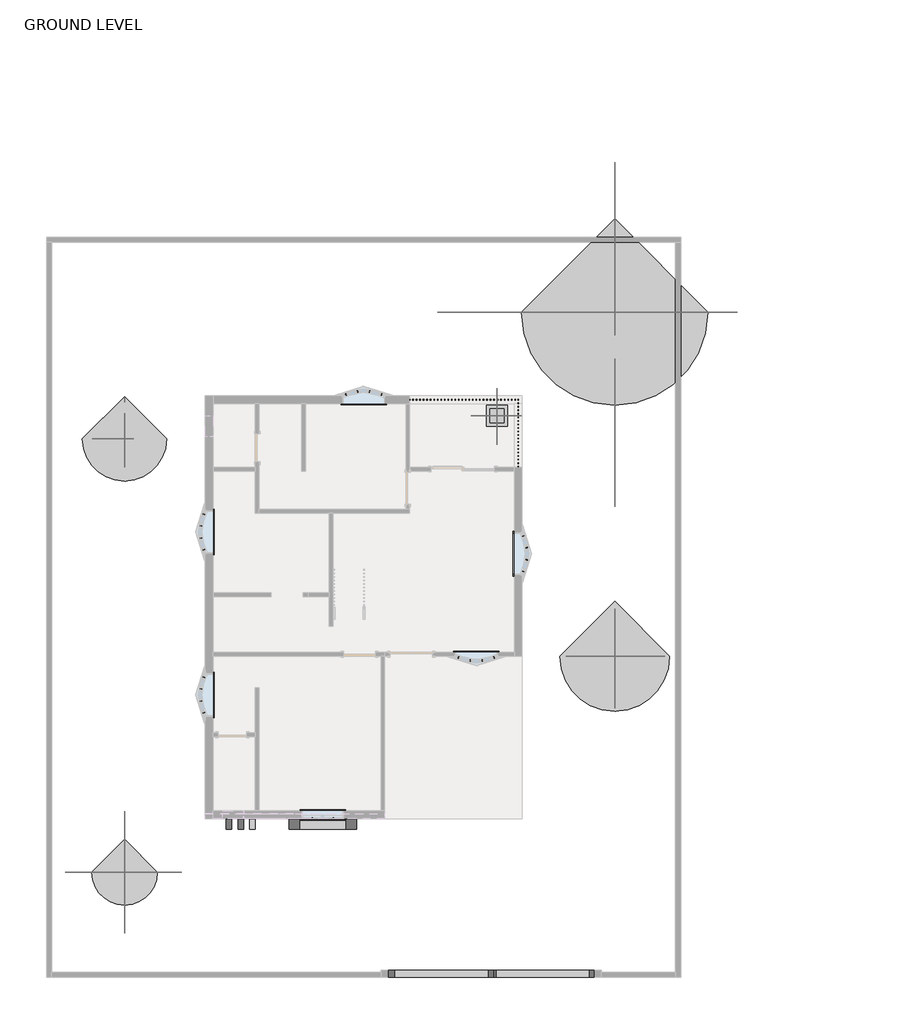
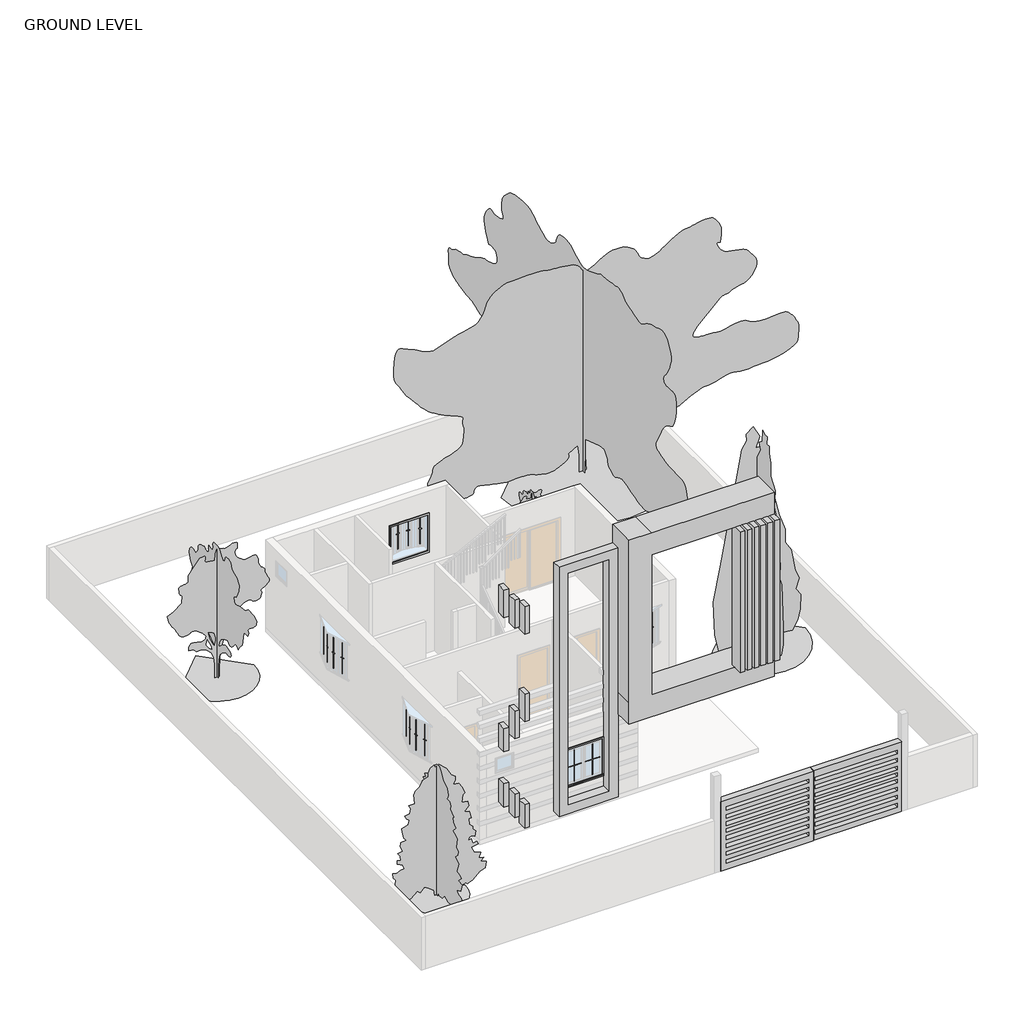
# One storey, part 3 of 3: 30 proxies, 6 geographic elements, 1 railing.
"""IFC4 building model written with IfcOpenShell, lengths in millimetres."""

from ifc_helpers import new_model, si_unit, frame, origin, place, context, project, spatial, polyline, outline, extrude, faceted_brep, transform, mapped, element, save
from components import generic_models_1_generic_models_1_2996b52b, muntin_pattern_2x2_muntin_pattern_2x2_750a293b, muntin_pattern_2x2_muntin_pattern_2x2_a9af9031, muntin_pattern_2x2_muntin_pattern_2x2_4dfeb3f3, muntin_pattern_2x2_muntin_pattern_2x2_e852a7e4, trim_window_exterior_flat_with_sill_7cfdd449, trim_window_interior_flat_picture_frame_ace0ae79, trim_window_interior_flat_picture_frame_f1e0b15b, planter_2_x2_da431093, rpc_tree_conifer_9825e489, rpc_tree_conifer_red_cedar_10_2_15f97043, rpc_tree_deciduous_15_10e6bd9b, rpc_tree_deciduous_japanese_cherry_15_720dba75, rpc_tree_deciduous_japanese_cherry_15_2_e499737d

model = new_model("IFC4")

# Units and contexts
model_context = context("Model", 3, world=origin())
ifc_project = project(units=[si_unit("LENGTHUNIT", "METRE", prefix="MILLI")], contexts=[model_context])

# Site, building, storey
site = spatial("IfcSite", under=ifc_project)
building = spatial("IfcBuilding", under=site)
storey = spatial("IfcBuildingStorey", under=building, Name="GROUND LEVEL", Elevation=0.0)

# Proxies
placement = place(None, origin())
generic_models_1_generic_models_1_shape = generic_models_1_generic_models_1_2996b52b(model_context)
element("IfcBuildingElementProxy", 1, Name="Generic Models 1 : Generic Models 1", ObjectType="Generic Models 1 : Generic Models 1", at=placement, inside=storey, context=model_context, shape_type="MappedRepresentation", body=[
    mapped(generic_models_1_generic_models_1_shape, transform((0.0, 0.0, 0.0), x_axis=(1.0, 0.0, 0.0), y_axis=(0.0, 1.0, 0.0), z_axis=(0.0, 0.0, 1.0))),
])
muntin_pattern_2x2_muntin_pattern_2x2_shape = muntin_pattern_2x2_muntin_pattern_2x2_750a293b(model_context)
element("IfcBuildingElementProxy", 2, Name="Muntin Pattern_2x2 : Muntin Pattern_2x2", ObjectType="Muntin Pattern_2x2 : Muntin Pattern_2x2", at=placement, inside=storey, context=model_context, shape_type="MappedRepresentation", body=[
    mapped(muntin_pattern_2x2_muntin_pattern_2x2_shape, transform((2505.3380176, -905.714627, 1114.3823709), x_axis=(-0.9396926207859141, -0.3420201433256534, 0.0), y_axis=(0.3420201433256534, -0.9396926207859141, 0.0), z_axis=(0.0, 0.0, 1.0))),
])
element("IfcBuildingElementProxy", 3, Name="Muntin Pattern_2x2 : Muntin Pattern_2x2", ObjectType="Muntin Pattern_2x2 : Muntin Pattern_2x2", at=placement, inside=storey, context=model_context, shape_type="MappedRepresentation", body=[
    mapped(muntin_pattern_2x2_muntin_pattern_2x2_shape, transform((1482.0289314, -905.714627, 1114.3823709), x_axis=(-0.939692620785903, 0.34202014332568337, 0.0), y_axis=(-0.34202014332568337, -0.939692620785903, 0.0), z_axis=(0.0, 0.0, 1.0))),
])
element("IfcBuildingElementProxy", 4, Name="Muntin Pattern_2x2 : Muntin Pattern_2x2", ObjectType="Muntin Pattern_2x2 : Muntin Pattern_2x2", at=placement, inside=storey, context=model_context, shape_type="MappedRepresentation", body=[
    mapped(muntin_pattern_2x2_muntin_pattern_2x2_shape, transform((2166.3285145, -996.5519495, 1114.3823709), x_axis=(-0.9848077530122118, -0.17364817766690924, 0.0), y_axis=(0.17364817766690924, -0.9848077530122118, 0.0), z_axis=(0.0, 0.0, 1.0))),
])
element("IfcBuildingElementProxy", 5, Name="Muntin Pattern_2x2 : Muntin Pattern_2x2", ObjectType="Muntin Pattern_2x2 : Muntin Pattern_2x2", at=placement, inside=storey, context=model_context, shape_type="MappedRepresentation", body=[
    mapped(muntin_pattern_2x2_muntin_pattern_2x2_shape, transform((-5861.4497338, -2499.7623237, 1114.3823709), x_axis=(-0.342020143325655, 0.9396926207859135, 0.0), y_axis=(-0.9396926207859135, -0.342020143325655, 0.0), z_axis=(0.0, 0.0, 1.0))),
])
element("IfcBuildingElementProxy", 6, Name="Muntin Pattern_2x2 : Muntin Pattern_2x2", ObjectType="Muntin Pattern_2x2 : Muntin Pattern_2x2", at=placement, inside=storey, context=model_context, shape_type="MappedRepresentation", body=[
    mapped(muntin_pattern_2x2_muntin_pattern_2x2_shape, transform((-5861.4497338, -1476.4532375, 1114.3823709), x_axis=(0.34202014332568176, 0.9396926207859035, 0.0), y_axis=(-0.9396926207859035, 0.34202014332568176, 0.0), z_axis=(0.0, 0.0, 1.0))),
])
element("IfcBuildingElementProxy", 7, Name="Muntin Pattern_2x2 : Muntin Pattern_2x2", ObjectType="Muntin Pattern_2x2 : Muntin Pattern_2x2", at=placement, inside=storey, context=model_context, shape_type="MappedRepresentation", body=[
    mapped(muntin_pattern_2x2_muntin_pattern_2x2_shape, transform((-5952.2870564, -2160.7528206, 1114.3823709), x_axis=(-0.1736481776669109, 0.9848077530122115, 0.0), y_axis=(-0.9848077530122115, -0.1736481776669109, 0.0), z_axis=(0.0, 0.0, 1.0))),
])
element("IfcBuildingElementProxy", 8, Name="Muntin Pattern_2x2 : Muntin Pattern_2x2", ObjectType="Muntin Pattern_2x2 : Muntin Pattern_2x2", at=placement, inside=storey, context=model_context, shape_type="MappedRepresentation", body=[
    mapped(muntin_pattern_2x2_muntin_pattern_2x2_shape, transform((-1766.8960515, 6668.4018239, 1114.3823709), x_axis=(0.9396926207859141, 0.3420201433256534, 0.0), y_axis=(-0.3420201433256534, 0.9396926207859141, 0.0), z_axis=(0.0, 0.0, 1.0))),
])
element("IfcBuildingElementProxy", 9, Name="Muntin Pattern_2x2 : Muntin Pattern_2x2", ObjectType="Muntin Pattern_2x2 : Muntin Pattern_2x2", at=placement, inside=storey, context=model_context, shape_type="MappedRepresentation", body=[
    mapped(muntin_pattern_2x2_muntin_pattern_2x2_shape, transform((-743.5869653, 6668.4018239, 1114.3823709), x_axis=(0.939692620785903, -0.34202014332568337, 0.0), y_axis=(0.34202014332568337, 0.939692620785903, 0.0), z_axis=(0.0, 0.0, 1.0))),
])
element("IfcBuildingElementProxy", 10, Name="Muntin Pattern_2x2 : Muntin Pattern_2x2", ObjectType="Muntin Pattern_2x2 : Muntin Pattern_2x2", at=placement, inside=storey, context=model_context, shape_type="MappedRepresentation", body=[
    mapped(muntin_pattern_2x2_muntin_pattern_2x2_shape, transform((-1427.8865484, 6759.2391465, 1114.3823709), x_axis=(0.9848077530122118, 0.1736481776669092, 0.0), y_axis=(-0.1736481776669092, 0.9848077530122118, 0.0), z_axis=(0.0, 0.0, 1.0))),
])
element("IfcBuildingElementProxy", 11, Name="Muntin Pattern_2x2 : Muntin Pattern_2x2", ObjectType="Muntin Pattern_2x2 : Muntin Pattern_2x2", at=placement, inside=storey, context=model_context, shape_type="MappedRepresentation", body=[
    mapped(muntin_pattern_2x2_muntin_pattern_2x2_shape, transform((-5861.4497338, 2196.9198574, 1114.3823709), x_axis=(-0.342020143325655, 0.9396926207859135, 0.0), y_axis=(-0.9396926207859135, -0.342020143325655, 0.0), z_axis=(0.0, 0.0, 1.0))),
])
element("IfcBuildingElementProxy", 12, Name="Muntin Pattern_2x2 : Muntin Pattern_2x2", ObjectType="Muntin Pattern_2x2 : Muntin Pattern_2x2", at=placement, inside=storey, context=model_context, shape_type="MappedRepresentation", body=[
    mapped(muntin_pattern_2x2_muntin_pattern_2x2_shape, transform((-5861.4497338, 3220.2289436, 1114.3823709), x_axis=(0.34202014332568176, 0.9396926207859035, 0.0), y_axis=(-0.9396926207859035, 0.34202014332568176, 0.0), z_axis=(0.0, 0.0, 1.0))),
])
element("IfcBuildingElementProxy", 13, Name="Muntin Pattern_2x2 : Muntin Pattern_2x2", ObjectType="Muntin Pattern_2x2 : Muntin Pattern_2x2", at=placement, inside=storey, context=model_context, shape_type="MappedRepresentation", body=[
    mapped(muntin_pattern_2x2_muntin_pattern_2x2_shape, transform((-5952.2870564, 2535.9293605, 1114.3823709), x_axis=(-0.1736481776669109, 0.9848077530122115, 0.0), y_axis=(-0.9848077530122115, -0.1736481776669109, 0.0), z_axis=(0.0, 0.0, 1.0))),
])
element("IfcBuildingElementProxy", 14, Name="Muntin Pattern_2x2 : Muntin Pattern_2x2", ObjectType="Muntin Pattern_2x2 : Muntin Pattern_2x2", at=placement, inside=storey, context=model_context, shape_type="MappedRepresentation", body=[
    mapped(muntin_pattern_2x2_muntin_pattern_2x2_shape, transform((3350.9667171, 2592.8981416, 730.25), x_axis=(0.34202014332565495, -0.9396926207859135, 0.0), y_axis=(0.9396926207859135, 0.34202014332565495, 0.0), z_axis=(0.0, 0.0, 1.0))),
])
element("IfcBuildingElementProxy", 15, Name="Muntin Pattern_2x2 : Muntin Pattern_2x2", ObjectType="Muntin Pattern_2x2 : Muntin Pattern_2x2", at=placement, inside=storey, context=model_context, shape_type="MappedRepresentation", body=[
    mapped(muntin_pattern_2x2_muntin_pattern_2x2_shape, transform((3350.9667171, 1569.5890554, 730.25), x_axis=(-0.3420201433256818, -0.9396926207859035, 0.0), y_axis=(0.9396926207859035, -0.3420201433256818, 0.0), z_axis=(0.0, 0.0, 1.0))),
])
element("IfcBuildingElementProxy", 16, Name="Muntin Pattern_2x2 : Muntin Pattern_2x2", ObjectType="Muntin Pattern_2x2 : Muntin Pattern_2x2", at=placement, inside=storey, context=model_context, shape_type="MappedRepresentation", body=[
    mapped(muntin_pattern_2x2_muntin_pattern_2x2_shape, transform((3441.8040397, 2253.8886385, 730.25), x_axis=(0.17364817766691085, -0.9848077530122115, 0.0), y_axis=(0.9848077530122115, 0.17364817766691085, 0.0), z_axis=(0.0, 0.0, 1.0))),
])
muntin_pattern_2x2_muntin_pattern_2x2_2_shape = muntin_pattern_2x2_muntin_pattern_2x2_a9af9031(model_context)
element("IfcBuildingElementProxy", 17, Name="Muntin Pattern_2x2 : Muntin Pattern_2x2", ObjectType="Muntin Pattern_2x2 : Muntin Pattern_2x2", at=placement, inside=storey, context=model_context, shape_type="MappedRepresentation", body=[
    mapped(muntin_pattern_2x2_muntin_pattern_2x2_2_shape, transform((1821.0384345, -996.5519495, 1114.3823709), x_axis=(0.9848077530122107, -0.17364817766691557, 0.0), y_axis=(0.17364817766691557, 0.9848077530122107, 0.0), z_axis=(0.0, 0.0, 1.0))),
])
element("IfcBuildingElementProxy", 18, Name="Muntin Pattern_2x2 : Muntin Pattern_2x2", ObjectType="Muntin Pattern_2x2 : Muntin Pattern_2x2", at=placement, inside=storey, context=model_context, shape_type="MappedRepresentation", body=[
    mapped(muntin_pattern_2x2_muntin_pattern_2x2_2_shape, transform((-5952.2870564, -1815.4627406, 1114.3823709), x_axis=(-0.1736481776669139, -0.984807753012211, 0.0), y_axis=(0.984807753012211, -0.1736481776669139, 0.0), z_axis=(0.0, 0.0, 1.0))),
])
element("IfcBuildingElementProxy", 19, Name="Muntin Pattern_2x2 : Muntin Pattern_2x2", ObjectType="Muntin Pattern_2x2 : Muntin Pattern_2x2", at=placement, inside=storey, context=model_context, shape_type="MappedRepresentation", body=[
    mapped(muntin_pattern_2x2_muntin_pattern_2x2_2_shape, transform((-1082.5964684, 6759.2391465, 1114.3823709), x_axis=(-0.9848077530122107, 0.1736481776669156, 0.0), y_axis=(-0.1736481776669156, -0.9848077530122107, 0.0), z_axis=(0.0, 0.0, 1.0))),
])
element("IfcBuildingElementProxy", 20, Name="Muntin Pattern_2x2 : Muntin Pattern_2x2", ObjectType="Muntin Pattern_2x2 : Muntin Pattern_2x2", at=placement, inside=storey, context=model_context, shape_type="MappedRepresentation", body=[
    mapped(muntin_pattern_2x2_muntin_pattern_2x2_2_shape, transform((-5952.2870564, 2881.2194405, 1114.3823709), x_axis=(-0.1736481776669139, -0.984807753012211, 0.0), y_axis=(0.984807753012211, -0.1736481776669139, 0.0), z_axis=(0.0, 0.0, 1.0))),
])
element("IfcBuildingElementProxy", 21, Name="Muntin Pattern_2x2 : Muntin Pattern_2x2", ObjectType="Muntin Pattern_2x2 : Muntin Pattern_2x2", at=placement, inside=storey, context=model_context, shape_type="MappedRepresentation", body=[
    mapped(muntin_pattern_2x2_muntin_pattern_2x2_2_shape, transform((3441.8040397, 1908.5985585, 730.25), x_axis=(0.17364817766691396, 0.984807753012211, 0.0), y_axis=(-0.984807753012211, 0.17364817766691396, 0.0), z_axis=(0.0, 0.0, 1.0))),
])
muntin_pattern_2x2_muntin_pattern_2x2_3_shape = muntin_pattern_2x2_muntin_pattern_2x2_4dfeb3f3(model_context)
element("IfcBuildingElementProxy", 22, Name="Muntin Pattern_2x2 : Muntin Pattern_2x2", ObjectType="Muntin Pattern_2x2 : Muntin Pattern_2x2", at=placement, inside=storey, context=model_context, shape_type="MappedRepresentation", body=[
    mapped(muntin_pattern_2x2_muntin_pattern_2x2_3_shape, transform((-2130.1595223, -5548.2814015, 984.25), x_axis=(-1.0, 0.0, 0.0), y_axis=(0.0, -1.0, 0.0), z_axis=(0.0, 0.0, 1.0))),
])
muntin_pattern_2x2_muntin_pattern_2x2_4_shape = muntin_pattern_2x2_muntin_pattern_2x2_e852a7e4(model_context)
element("IfcBuildingElementProxy", 23, Name="Muntin Pattern_2x2 : Muntin Pattern_2x2", ObjectType="Muntin Pattern_2x2 : Muntin Pattern_2x2", at=placement, inside=storey, context=model_context, shape_type="MappedRepresentation", body=[
    mapped(muntin_pattern_2x2_muntin_pattern_2x2_4_shape, transform((-2736.5845223, -5548.2814015, 984.25), x_axis=(1.0, 0.0, 0.0), y_axis=(0.0, 1.0, 0.0), z_axis=(0.0, 0.0, 1.0))),
])
trim_window_exterior_flat_with_sill_shape = trim_window_exterior_flat_with_sill_7cfdd449(model_context)
element("IfcBuildingElementProxy", 24, Name="Trim-Window-Exterior-Flat : with Sill", ObjectType="Trim-Window-Exterior-Flat : with Sill", at=placement, inside=storey, context=model_context, shape_type="MappedRepresentation", body=[
    mapped(trim_window_exterior_flat_with_sill_shape, transform((-2433.3720223, -5557.8064015, 2133.6), x_axis=(1.0, 0.0, 0.0), y_axis=(0.0, 0.0, 1.0), z_axis=(0.0, -1.0, 0.0))),
])
trim_window_interior_flat_picture_frame_shape = trim_window_interior_flat_picture_frame_ace0ae79(model_context)
element("IfcBuildingElementProxy", 25, Name="Trim-Window-Interior-Flat : Picture Frame", ObjectType="Trim-Window-Interior-Flat : Picture Frame", at=placement, inside=storey, context=model_context, shape_type="MappedRepresentation", body=[
    mapped(trim_window_interior_flat_picture_frame_shape, transform((1993.6834745, -757.2064015, 2263.7323709), x_axis=(-1.0, 0.0, 0.0), y_axis=(0.0, 0.0, 1.0), z_axis=(0.0, 1.0, 0.0))),
])
element("IfcBuildingElementProxy", 26, Name="Trim-Window-Interior-Flat : Picture Frame", ObjectType="Trim-Window-Interior-Flat : Picture Frame", at=placement, inside=storey, context=model_context, shape_type="MappedRepresentation", body=[
    mapped(trim_window_interior_flat_picture_frame_shape, transform((-5598.6415084, -1988.1077806, 2263.7323709), x_axis=(0.0, 1.0, 0.0), y_axis=(0.0, 0.0, 1.0), z_axis=(1.0, 0.0, 0.0))),
])
element("IfcBuildingElementProxy", 27, Name="Trim-Window-Interior-Flat : Picture Frame", ObjectType="Trim-Window-Interior-Flat : Picture Frame", at=placement, inside=storey, context=model_context, shape_type="MappedRepresentation", body=[
    mapped(trim_window_interior_flat_picture_frame_shape, transform((-1255.2415084, 6405.5935985, 2263.7323709), x_axis=(1.0, 0.0, 0.0), y_axis=(0.0, 0.0, 1.0), z_axis=(0.0, -1.0, 0.0))),
])
element("IfcBuildingElementProxy", 28, Name="Trim-Window-Interior-Flat : Picture Frame", ObjectType="Trim-Window-Interior-Flat : Picture Frame", at=placement, inside=storey, context=model_context, shape_type="MappedRepresentation", body=[
    mapped(trim_window_interior_flat_picture_frame_shape, transform((-5598.6415084, 2708.5744005, 2263.7323709), x_axis=(0.0, 1.0, 0.0), y_axis=(0.0, 0.0, 1.0), z_axis=(1.0, 0.0, 0.0))),
])
element("IfcBuildingElementProxy", 29, Name="Trim-Window-Interior-Flat : Picture Frame", ObjectType="Trim-Window-Interior-Flat : Picture Frame", at=placement, inside=storey, context=model_context, shape_type="MappedRepresentation", body=[
    mapped(trim_window_interior_flat_picture_frame_shape, transform((3088.1584916, 2081.2435985, 1879.6), x_axis=(0.0, -1.0, 0.0), y_axis=(0.0, 0.0, 1.0), z_axis=(-1.0, 0.0, 0.0))),
])
trim_window_interior_flat_picture_frame_2_shape = trim_window_interior_flat_picture_frame_f1e0b15b(model_context)
element("IfcBuildingElementProxy", 30, Name="Trim-Window-Interior-Flat : Picture Frame", ObjectType="Trim-Window-Interior-Flat : Picture Frame", at=placement, inside=storey, context=model_context, shape_type="MappedRepresentation", body=[
    mapped(trim_window_interior_flat_picture_frame_2_shape, transform((-2433.3720223, -5329.2064015, 2133.6), x_axis=(-1.0, 0.0, 0.0), y_axis=(0.0, 0.0, 1.0), z_axis=(0.0, 1.0, 0.0))),
])

# Geographic elements
planter_2_x2_shape = planter_2_x2_da431093(model_context)
element("IfcGeographicElement", 31, ObjectType="Planter : 2'x2'", at=placement, inside=storey, context=model_context, shape_type="MappedRepresentation", body=[
    mapped(planter_2_x2_shape, transform((2592.8584916, 6062.6935985, 0.0), x_axis=(1.0, 0.0, 0.0), y_axis=(0.0, 1.0, 0.0), z_axis=(0.0, 0.0, 1.0))),
])
rpc_tree_conifer_shape = rpc_tree_conifer_9825e489(model_context)
element("IfcGeographicElement", 32, ObjectType="RPC Tree - Conifer", at=placement, inside=storey, context=model_context, shape_type="MappedRepresentation", body=[
    mapped(rpc_tree_conifer_shape, transform((-8151.5381795, -7100.8564015, -152.4), x_axis=(1.0, 0.0, 0.0), y_axis=(0.0, 1.0, 0.0), z_axis=(0.0, 0.0, 1.0))),
])
rpc_tree_conifer_red_cedar_10_2_shape = rpc_tree_conifer_red_cedar_10_2_15f97043(model_context)
element("IfcGeographicElement", 33, ObjectType="RPC Tree - Conifer : Red Cedar - 10' 2", at=placement, inside=storey, context=model_context, shape_type="MappedRepresentation", body=[
    mapped(rpc_tree_conifer_red_cedar_10_2_shape, transform((5983.5618205, -871.5064015, -152.4), x_axis=(1.0, 0.0, 0.0), y_axis=(0.0, 1.0, 0.0), z_axis=(0.0, 0.0, 1.0))),
])
rpc_tree_deciduous_15_shape = rpc_tree_deciduous_15_10e6bd9b(model_context)
element("IfcGeographicElement", 34, ObjectType="RPC Tree - Deciduous : 15'", at=placement, inside=storey, context=model_context, shape_type="MappedRepresentation", body=[
    mapped(rpc_tree_deciduous_15_shape, transform((5983.7584916, 9047.1935985, -152.4), x_axis=(1.0, 0.0, 0.0), y_axis=(0.0, 1.0, 0.0), z_axis=(0.0, 0.0, 1.0))),
])
rpc_tree_deciduous_japanese_cherry_15_shape = rpc_tree_deciduous_japanese_cherry_15_720dba75(model_context)
element("IfcGeographicElement", 35, ObjectType="RPC Tree - Deciduous : Japanese Cherry - 15'", at=placement, inside=storey, context=model_context, shape_type="MappedRepresentation", body=[
    mapped(rpc_tree_deciduous_japanese_cherry_15_shape, transform((2592.8584916, 6062.6935985, 0.0), x_axis=(1.0, 0.0, 0.0), y_axis=(0.0, 1.0, 0.0), z_axis=(0.0, 0.0, 1.0))),
])
rpc_tree_deciduous_japanese_cherry_15_2_shape = rpc_tree_deciduous_japanese_cherry_15_2_e499737d(model_context)
element("IfcGeographicElement", 36, ObjectType="RPC Tree - Deciduous : Japanese Cherry - 15' 2", at=placement, inside=storey, context=model_context, shape_type="MappedRepresentation", body=[
    mapped(rpc_tree_deciduous_japanese_cherry_15_2_shape, transform((-8151.3415084, 5389.5935985, -152.4), x_axis=(1.0, 0.0, 0.0), y_axis=(0.0, 1.0, 0.0), z_axis=(0.0, 0.0, 1.0))),
])

# Railing
element("IfcRailing", 37, ObjectType="Handrail - Rectangular", at=placement, inside=storey, context=model_context, shape_type="SolidModel", body=[
    faceted_brep([(65.5584916, 6545.2935985, 1371.6), (65.5584916, 6545.2935985, 1320.8), (65.5584916, 6494.4935985, 1320.8), (65.5584916, 6494.4935985, 1371.6), (3227.8584916, 6545.2935985, 1371.6), (3227.8584916, 6545.2935985, 1320.8), (3177.0584916, 6494.4935985, 1320.8), (3177.0584916, 6494.4935985, 1371.6), (3227.8584916, 4576.7935985, 1371.6), (3177.0584916, 4576.7935985, 1371.6), (3177.0584916, 4576.7935985, 1320.8), (3227.8584916, 4576.7935985, 1320.8)], [[[0, 1, 2, 3]], [[1, 0, 4, 5]], [[2, 1, 5, 6]], [[3, 2, 6, 7]], [[0, 3, 7, 4]], [[8, 9, 10, 11]], [[5, 4, 8, 11]], [[6, 5, 11, 10]], [[7, 6, 10, 9]], [[4, 7, 9, 8]]]),
    extrude(outline(polyline([(3192.9334916, 4599.0185985), (3211.9834916, 4599.0185985), (3211.9834916, 4579.9685985), (3192.9334916, 4579.9685985), (3192.9334916, 4599.0185985)])), frame((0.0, 0.0, 609.6), z_axis=(0.0, 0.0, 1.0), x_axis=(1.0, 0.0, 0.0)), (0.0, 0.0, 1.0), 711.2),
    extrude(outline(polyline([(3192.9334916, 4700.6185985), (3211.9834916, 4700.6185985), (3211.9834916, 4681.5685985), (3192.9334916, 4681.5685985), (3192.9334916, 4700.6185985)])), frame((0.0, 0.0, 609.6), z_axis=(0.0, 0.0, 1.0), x_axis=(1.0, 0.0, 0.0)), (0.0, 0.0, 1.0), 711.2),
    extrude(outline(polyline([(3192.9334916, 4802.2185985), (3211.9834916, 4802.2185985), (3211.9834916, 4783.1685985), (3192.9334916, 4783.1685985), (3192.9334916, 4802.2185985)])), frame((0.0, 0.0, 609.6), z_axis=(0.0, 0.0, 1.0), x_axis=(1.0, 0.0, 0.0)), (0.0, 0.0, 1.0), 711.2),
    extrude(outline(polyline([(3192.9334916, 4903.8185985), (3211.9834916, 4903.8185985), (3211.9834916, 4884.7685985), (3192.9334916, 4884.7685985), (3192.9334916, 4903.8185985)])), frame((0.0, 0.0, 609.6), z_axis=(0.0, 0.0, 1.0), x_axis=(1.0, 0.0, 0.0)), (0.0, 0.0, 1.0), 711.2),
    extrude(outline(polyline([(3192.9334916, 5005.4185985), (3211.9834916, 5005.4185985), (3211.9834916, 4986.3685985), (3192.9334916, 4986.3685985), (3192.9334916, 5005.4185985)])), frame((0.0, 0.0, 609.6), z_axis=(0.0, 0.0, 1.0), x_axis=(1.0, 0.0, 0.0)), (0.0, 0.0, 1.0), 711.2),
    extrude(outline(polyline([(3192.9334916, 5107.0185985), (3211.9834916, 5107.0185985), (3211.9834916, 5087.9685985), (3192.9334916, 5087.9685985), (3192.9334916, 5107.0185985)])), frame((0.0, 0.0, 609.6), z_axis=(0.0, 0.0, 1.0), x_axis=(1.0, 0.0, 0.0)), (0.0, 0.0, 1.0), 711.2),
    extrude(outline(polyline([(3192.9334916, 5208.6185985), (3211.9834916, 5208.6185985), (3211.9834916, 5189.5685985), (3192.9334916, 5189.5685985), (3192.9334916, 5208.6185985)])), frame((0.0, 0.0, 609.6), z_axis=(0.0, 0.0, 1.0), x_axis=(1.0, 0.0, 0.0)), (0.0, 0.0, 1.0), 711.2),
    extrude(outline(polyline([(3192.9334916, 5310.2185985), (3211.9834916, 5310.2185985), (3211.9834916, 5291.1685985), (3192.9334916, 5291.1685985), (3192.9334916, 5310.2185985)])), frame((0.0, 0.0, 609.6), z_axis=(0.0, 0.0, 1.0), x_axis=(1.0, 0.0, 0.0)), (0.0, 0.0, 1.0), 711.2),
    extrude(outline(polyline([(3192.9334916, 5411.8185985), (3211.9834916, 5411.8185985), (3211.9834916, 5392.7685985), (3192.9334916, 5392.7685985), (3192.9334916, 5411.8185985)])), frame((0.0, 0.0, 609.6), z_axis=(0.0, 0.0, 1.0), x_axis=(1.0, 0.0, 0.0)), (0.0, 0.0, 1.0), 711.2),
    extrude(outline(polyline([(3192.9334916, 5513.4185985), (3211.9834916, 5513.4185985), (3211.9834916, 5494.3685985), (3192.9334916, 5494.3685985), (3192.9334916, 5513.4185985)])), frame((0.0, 0.0, 609.6), z_axis=(0.0, 0.0, 1.0), x_axis=(1.0, 0.0, 0.0)), (0.0, 0.0, 1.0), 711.2),
    extrude(outline(polyline([(3192.9334916, 5615.0185985), (3211.9834916, 5615.0185985), (3211.9834916, 5595.9685985), (3192.9334916, 5595.9685985), (3192.9334916, 5615.0185985)])), frame((0.0, 0.0, 609.6), z_axis=(0.0, 0.0, 1.0), x_axis=(1.0, 0.0, 0.0)), (0.0, 0.0, 1.0), 711.2),
    extrude(outline(polyline([(3192.9334916, 5716.6185985), (3211.9834916, 5716.6185985), (3211.9834916, 5697.5685985), (3192.9334916, 5697.5685985), (3192.9334916, 5716.6185985)])), frame((0.0, 0.0, 609.6), z_axis=(0.0, 0.0, 1.0), x_axis=(1.0, 0.0, 0.0)), (0.0, 0.0, 1.0), 711.2),
    extrude(outline(polyline([(3192.9334916, 5818.2185985), (3211.9834916, 5818.2185985), (3211.9834916, 5799.1685985), (3192.9334916, 5799.1685985), (3192.9334916, 5818.2185985)])), frame((0.0, 0.0, 609.6), z_axis=(0.0, 0.0, 1.0), x_axis=(1.0, 0.0, 0.0)), (0.0, 0.0, 1.0), 711.2),
    extrude(outline(polyline([(3192.9334916, 5919.8185985), (3211.9834916, 5919.8185985), (3211.9834916, 5900.7685985), (3192.9334916, 5900.7685985), (3192.9334916, 5919.8185985)])), frame((0.0, 0.0, 609.6), z_axis=(0.0, 0.0, 1.0), x_axis=(1.0, 0.0, 0.0)), (0.0, 0.0, 1.0), 711.2),
    extrude(outline(polyline([(3192.9334916, 6021.4185985), (3211.9834916, 6021.4185985), (3211.9834916, 6002.3685985), (3192.9334916, 6002.3685985), (3192.9334916, 6021.4185985)])), frame((0.0, 0.0, 609.6), z_axis=(0.0, 0.0, 1.0), x_axis=(1.0, 0.0, 0.0)), (0.0, 0.0, 1.0), 711.2),
    extrude(outline(polyline([(3192.9334916, 6123.0185985), (3211.9834916, 6123.0185985), (3211.9834916, 6103.9685985), (3192.9334916, 6103.9685985), (3192.9334916, 6123.0185985)])), frame((0.0, 0.0, 609.6), z_axis=(0.0, 0.0, 1.0), x_axis=(1.0, 0.0, 0.0)), (0.0, 0.0, 1.0), 711.2),
    extrude(outline(polyline([(3192.9334916, 6224.6185985), (3211.9834916, 6224.6185985), (3211.9834916, 6205.5685985), (3192.9334916, 6205.5685985), (3192.9334916, 6224.6185985)])), frame((0.0, 0.0, 609.6), z_axis=(0.0, 0.0, 1.0), x_axis=(1.0, 0.0, 0.0)), (0.0, 0.0, 1.0), 711.2),
    extrude(outline(polyline([(3192.9334916, 6326.2185985), (3211.9834916, 6326.2185985), (3211.9834916, 6307.1685985), (3192.9334916, 6307.1685985), (3192.9334916, 6326.2185985)])), frame((0.0, 0.0, 609.6), z_axis=(0.0, 0.0, 1.0), x_axis=(1.0, 0.0, 0.0)), (0.0, 0.0, 1.0), 711.2),
    extrude(outline(polyline([(3192.9334916, 6427.8185985), (3211.9834916, 6427.8185985), (3211.9834916, 6408.7685985), (3192.9334916, 6408.7685985), (3192.9334916, 6427.8185985)])), frame((0.0, 0.0, 609.6), z_axis=(0.0, 0.0, 1.0), x_axis=(1.0, 0.0, 0.0)), (0.0, 0.0, 1.0), 711.2),
    extrude(outline(polyline([(3104.0334916, 6510.3685985), (3104.0334916, 6529.4185985), (3123.0834916, 6529.4185985), (3123.0834916, 6510.3685985), (3104.0334916, 6510.3685985)])), frame((0.0, 0.0, 609.6), z_axis=(0.0, 0.0, 1.0), x_axis=(1.0, 0.0, 0.0)), (0.0, 0.0, 1.0), 711.2),
    extrude(outline(polyline([(3002.4334916, 6510.3685985), (3002.4334916, 6529.4185985), (3021.4834916, 6529.4185985), (3021.4834916, 6510.3685985), (3002.4334916, 6510.3685985)])), frame((0.0, 0.0, 609.6), z_axis=(0.0, 0.0, 1.0), x_axis=(1.0, 0.0, 0.0)), (0.0, 0.0, 1.0), 711.2),
    extrude(outline(polyline([(2900.8334916, 6510.3685985), (2900.8334916, 6529.4185985), (2919.8834916, 6529.4185985), (2919.8834916, 6510.3685985), (2900.8334916, 6510.3685985)])), frame((0.0, 0.0, 609.6), z_axis=(0.0, 0.0, 1.0), x_axis=(1.0, 0.0, 0.0)), (0.0, 0.0, 1.0), 711.2),
    extrude(outline(polyline([(2799.2334916, 6510.3685985), (2799.2334916, 6529.4185985), (2818.2834916, 6529.4185985), (2818.2834916, 6510.3685985), (2799.2334916, 6510.3685985)])), frame((0.0, 0.0, 609.6), z_axis=(0.0, 0.0, 1.0), x_axis=(1.0, 0.0, 0.0)), (0.0, 0.0, 1.0), 711.2),
    extrude(outline(polyline([(2697.6334916, 6510.3685985), (2697.6334916, 6529.4185985), (2716.6834916, 6529.4185985), (2716.6834916, 6510.3685985), (2697.6334916, 6510.3685985)])), frame((0.0, 0.0, 609.6), z_axis=(0.0, 0.0, 1.0), x_axis=(1.0, 0.0, 0.0)), (0.0, 0.0, 1.0), 711.2),
    extrude(outline(polyline([(2596.0334916, 6510.3685985), (2596.0334916, 6529.4185985), (2615.0834916, 6529.4185985), (2615.0834916, 6510.3685985), (2596.0334916, 6510.3685985)])), frame((0.0, 0.0, 609.6), z_axis=(0.0, 0.0, 1.0), x_axis=(1.0, 0.0, 0.0)), (0.0, 0.0, 1.0), 711.2),
    extrude(outline(polyline([(2494.4334916, 6510.3685985), (2494.4334916, 6529.4185985), (2513.4834916, 6529.4185985), (2513.4834916, 6510.3685985), (2494.4334916, 6510.3685985)])), frame((0.0, 0.0, 609.6), z_axis=(0.0, 0.0, 1.0), x_axis=(1.0, 0.0, 0.0)), (0.0, 0.0, 1.0), 711.2),
    extrude(outline(polyline([(2392.8334916, 6510.3685985), (2392.8334916, 6529.4185985), (2411.8834916, 6529.4185985), (2411.8834916, 6510.3685985), (2392.8334916, 6510.3685985)])), frame((0.0, 0.0, 609.6), z_axis=(0.0, 0.0, 1.0), x_axis=(1.0, 0.0, 0.0)), (0.0, 0.0, 1.0), 711.2),
    extrude(outline(polyline([(2291.2334916, 6510.3685985), (2291.2334916, 6529.4185985), (2310.2834916, 6529.4185985), (2310.2834916, 6510.3685985), (2291.2334916, 6510.3685985)])), frame((0.0, 0.0, 609.6), z_axis=(0.0, 0.0, 1.0), x_axis=(1.0, 0.0, 0.0)), (0.0, 0.0, 1.0), 711.2),
    extrude(outline(polyline([(2189.6334916, 6510.3685985), (2189.6334916, 6529.4185985), (2208.6834916, 6529.4185985), (2208.6834916, 6510.3685985), (2189.6334916, 6510.3685985)])), frame((0.0, 0.0, 609.6), z_axis=(0.0, 0.0, 1.0), x_axis=(1.0, 0.0, 0.0)), (0.0, 0.0, 1.0), 711.2),
    extrude(outline(polyline([(2088.0334916, 6510.3685985), (2088.0334916, 6529.4185985), (2107.0834916, 6529.4185985), (2107.0834916, 6510.3685985), (2088.0334916, 6510.3685985)])), frame((0.0, 0.0, 609.6), z_axis=(0.0, 0.0, 1.0), x_axis=(1.0, 0.0, 0.0)), (0.0, 0.0, 1.0), 711.2),
    extrude(outline(polyline([(1986.4334916, 6510.3685985), (1986.4334916, 6529.4185985), (2005.4834916, 6529.4185985), (2005.4834916, 6510.3685985), (1986.4334916, 6510.3685985)])), frame((0.0, 0.0, 609.6), z_axis=(0.0, 0.0, 1.0), x_axis=(1.0, 0.0, 0.0)), (0.0, 0.0, 1.0), 711.2),
    extrude(outline(polyline([(1884.8334916, 6510.3685985), (1884.8334916, 6529.4185985), (1903.8834916, 6529.4185985), (1903.8834916, 6510.3685985), (1884.8334916, 6510.3685985)])), frame((0.0, 0.0, 609.6), z_axis=(0.0, 0.0, 1.0), x_axis=(1.0, 0.0, 0.0)), (0.0, 0.0, 1.0), 711.2),
    extrude(outline(polyline([(1783.2334916, 6510.3685985), (1783.2334916, 6529.4185985), (1802.2834916, 6529.4185985), (1802.2834916, 6510.3685985), (1783.2334916, 6510.3685985)])), frame((0.0, 0.0, 609.6), z_axis=(0.0, 0.0, 1.0), x_axis=(1.0, 0.0, 0.0)), (0.0, 0.0, 1.0), 711.2),
    extrude(outline(polyline([(1681.6334916, 6510.3685985), (1681.6334916, 6529.4185985), (1700.6834916, 6529.4185985), (1700.6834916, 6510.3685985), (1681.6334916, 6510.3685985)])), frame((0.0, 0.0, 609.6), z_axis=(0.0, 0.0, 1.0), x_axis=(1.0, 0.0, 0.0)), (0.0, 0.0, 1.0), 711.2),
    extrude(outline(polyline([(1580.0334916, 6510.3685985), (1580.0334916, 6529.4185985), (1599.0834916, 6529.4185985), (1599.0834916, 6510.3685985), (1580.0334916, 6510.3685985)])), frame((0.0, 0.0, 609.6), z_axis=(0.0, 0.0, 1.0), x_axis=(1.0, 0.0, 0.0)), (0.0, 0.0, 1.0), 711.2),
    extrude(outline(polyline([(1478.4334916, 6510.3685985), (1478.4334916, 6529.4185985), (1497.4834916, 6529.4185985), (1497.4834916, 6510.3685985), (1478.4334916, 6510.3685985)])), frame((0.0, 0.0, 609.6), z_axis=(0.0, 0.0, 1.0), x_axis=(1.0, 0.0, 0.0)), (0.0, 0.0, 1.0), 711.2),
    extrude(outline(polyline([(1376.8334916, 6510.3685985), (1376.8334916, 6529.4185985), (1395.8834916, 6529.4185985), (1395.8834916, 6510.3685985), (1376.8334916, 6510.3685985)])), frame((0.0, 0.0, 609.6), z_axis=(0.0, 0.0, 1.0), x_axis=(1.0, 0.0, 0.0)), (0.0, 0.0, 1.0), 711.2),
    extrude(outline(polyline([(1275.2334916, 6510.3685985), (1275.2334916, 6529.4185985), (1294.2834916, 6529.4185985), (1294.2834916, 6510.3685985), (1275.2334916, 6510.3685985)])), frame((0.0, 0.0, 609.6), z_axis=(0.0, 0.0, 1.0), x_axis=(1.0, 0.0, 0.0)), (0.0, 0.0, 1.0), 711.2),
    extrude(outline(polyline([(1173.6334916, 6510.3685985), (1173.6334916, 6529.4185985), (1192.6834916, 6529.4185985), (1192.6834916, 6510.3685985), (1173.6334916, 6510.3685985)])), frame((0.0, 0.0, 609.6), z_axis=(0.0, 0.0, 1.0), x_axis=(1.0, 0.0, 0.0)), (0.0, 0.0, 1.0), 711.2),
    extrude(outline(polyline([(1072.0334916, 6510.3685985), (1072.0334916, 6529.4185985), (1091.0834916, 6529.4185985), (1091.0834916, 6510.3685985), (1072.0334916, 6510.3685985)])), frame((0.0, 0.0, 609.6), z_axis=(0.0, 0.0, 1.0), x_axis=(1.0, 0.0, 0.0)), (0.0, 0.0, 1.0), 711.2),
    extrude(outline(polyline([(970.4334916, 6510.3685985), (970.4334916, 6529.4185985), (989.4834916, 6529.4185985), (989.4834916, 6510.3685985), (970.4334916, 6510.3685985)])), frame((0.0, 0.0, 609.6), z_axis=(0.0, 0.0, 1.0), x_axis=(1.0, 0.0, 0.0)), (0.0, 0.0, 1.0), 711.2),
    extrude(outline(polyline([(868.8334916, 6510.3685985), (868.8334916, 6529.4185985), (887.8834916, 6529.4185985), (887.8834916, 6510.3685985), (868.8334916, 6510.3685985)])), frame((0.0, 0.0, 609.6), z_axis=(0.0, 0.0, 1.0), x_axis=(1.0, 0.0, 0.0)), (0.0, 0.0, 1.0), 711.2),
    extrude(outline(polyline([(767.2334916, 6510.3685985), (767.2334916, 6529.4185985), (786.2834916, 6529.4185985), (786.2834916, 6510.3685985), (767.2334916, 6510.3685985)])), frame((0.0, 0.0, 609.6), z_axis=(0.0, 0.0, 1.0), x_axis=(1.0, 0.0, 0.0)), (0.0, 0.0, 1.0), 711.2),
    extrude(outline(polyline([(665.6334916, 6510.3685985), (665.6334916, 6529.4185985), (684.6834916, 6529.4185985), (684.6834916, 6510.3685985), (665.6334916, 6510.3685985)])), frame((0.0, 0.0, 609.6), z_axis=(0.0, 0.0, 1.0), x_axis=(1.0, 0.0, 0.0)), (0.0, 0.0, 1.0), 711.2),
    extrude(outline(polyline([(564.0334916, 6510.3685985), (564.0334916, 6529.4185985), (583.0834916, 6529.4185985), (583.0834916, 6510.3685985), (564.0334916, 6510.3685985)])), frame((0.0, 0.0, 609.6), z_axis=(0.0, 0.0, 1.0), x_axis=(1.0, 0.0, 0.0)), (0.0, 0.0, 1.0), 711.2),
    extrude(outline(polyline([(462.4334916, 6510.3685985), (462.4334916, 6529.4185985), (481.4834916, 6529.4185985), (481.4834916, 6510.3685985), (462.4334916, 6510.3685985)])), frame((0.0, 0.0, 609.6), z_axis=(0.0, 0.0, 1.0), x_axis=(1.0, 0.0, 0.0)), (0.0, 0.0, 1.0), 711.2),
    extrude(outline(polyline([(360.8334916, 6510.3685985), (360.8334916, 6529.4185985), (379.8834916, 6529.4185985), (379.8834916, 6510.3685985), (360.8334916, 6510.3685985)])), frame((0.0, 0.0, 609.6), z_axis=(0.0, 0.0, 1.0), x_axis=(1.0, 0.0, 0.0)), (0.0, 0.0, 1.0), 711.2),
    extrude(outline(polyline([(259.2334916, 6510.3685985), (259.2334916, 6529.4185985), (278.2834916, 6529.4185985), (278.2834916, 6510.3685985), (259.2334916, 6510.3685985)])), frame((0.0, 0.0, 609.6), z_axis=(0.0, 0.0, 1.0), x_axis=(1.0, 0.0, 0.0)), (0.0, 0.0, 1.0), 711.2),
    extrude(outline(polyline([(157.6334916, 6510.3685985), (157.6334916, 6529.4185985), (176.6834916, 6529.4185985), (176.6834916, 6510.3685985), (157.6334916, 6510.3685985)])), frame((0.0, 0.0, 609.6), z_axis=(0.0, 0.0, 1.0), x_axis=(1.0, 0.0, 0.0)), (0.0, 0.0, 1.0), 711.2),
    extrude(outline(polyline([(3192.9334916, 6510.3685985), (3192.9334916, 6529.4185985), (3211.9834916, 6529.4185985), (3211.9834916, 6510.3685985), (3192.9334916, 6510.3685985)])), frame((0.0, 0.0, 609.6), z_axis=(0.0, 0.0, 1.0), x_axis=(1.0, 0.0, 0.0)), (0.0, 0.0, 1.0), 711.2),
    extrude(outline(polyline([(3192.9334916, 4595.8435985), (3211.9834916, 4595.8435985), (3211.9834916, 4576.7935985), (3192.9334916, 4576.7935985), (3192.9334916, 4595.8435985)])), frame((0.0, 0.0, 609.6), z_axis=(0.0, 0.0, 1.0), x_axis=(1.0, 0.0, 0.0)), (0.0, 0.0, 1.0), 711.2),
    extrude(outline(polyline([(65.5584916, 6510.3685985), (65.5584916, 6529.4185985), (84.6084916, 6529.4185985), (84.6084916, 6510.3685985), (65.5584916, 6510.3685985)])), frame((0.0, 0.0, 609.6), z_axis=(0.0, 0.0, 1.0), x_axis=(1.0, 0.0, 0.0)), (0.0, 0.0, 1.0), 711.2),
])

save(model, "model.ifc")

# Revit data of these elements
# Type "Muntin Pattern_2x2 : Muntin Pattern_2x2"
#   Width [instance default] = 4' - 0"
#   Thickness = 0' - 0 1/2"
#   Height [instance default] = 4' - 0"
#   Distance = 0' - 0 3/4"
#   Interior Material [instance default] = none
#   Exterior Material [instance default] = none
#   Default Elevation = 0
# Type "Trim-Window-Exterior-Flat : with Sill"
#   Trim Width = 0' - 2 1/4"
#   Trim Thickness_Picture Frame = 0' - 1 1/4"
#   Trim Thickness_with Sill = 0' - 0 3/4"
#   Sill Thickness = 0' - 1 1/4"
#   Opening Width [instance default] = 2' - 0"
#   Opening Height [instance default] = 3' - 0"
#   Default Elevation = 4' - 0"
#   Sill = yes
#   Picture Frame = no
#   Trim Material [instance default] = none
# Type "Trim-Window-Interior-Flat : Picture Frame"
#   Trim Thickness_Picture Frame = 0' - 1 1/4"
#   Trim Width = 0' - 2 1/4"
#   Trim Thickness_with Sill = 0' - 0 3/4"
#   Sill Thickness = 0' - 1 1/4"
#   Opening Width [instance default] = 2' - 0"
#   Opening Height [instance default] = 3' - 0"
#   Default Elevation = 4' - 0"
#   Sill = no
#   Picture Frame = yes
#   Trim Material [instance default] = none
# Type "Planter : 2'x2'"
#   Depth = 2' - 0"
#   Height = 2' - 0"
#   Width = 2' - 0"
#   Material = Concrete, Precast
# Type "RPC Tree - Conifer"
#   built-in parameter 1005198 = "{2, 15},{39, RPC-16-G0M4-N9PX-U6TN-C000-ST1L-LVER-AU},{1, 0},{1, 0},{2, 35},{1, 8},{5, Color},{1, 0},{1, 0},{3, 0.8},{3, 0.8},{3, 0.8},{1, 8},{7, BBoxMin},{1, 0},{1, 0},{1, 0},{1, 0},{1, 0},{1, 8},{7, BBoxMax},{1, 0},{1, 0},{1, 0},{1, 0},{1, 0},{2, 11},{9, RPCTypeId},{1, 0},{1, 0},{39, RPC-16-G0M4-N9PX-U6TN-C000-ST1L-LVER-AU},{1, 6},{14, RPCPlantHeight},{1, 0},{1, 0},{2, 13},{2, 11},{7, keyword},{1, 0},{1, 0},{91, :Geometry:RPC:Colorado Spruce:colorado spruce:pinaceae:picea:pungens:evergreen:conifer:blue},{2, 11},{8, category},{1, 0},{1, 0},{16, :Trees [General]},{2, 11},{12, LocalizedUID},{1, 0},{1, 0},{15, Colorado Spruce},{2, 14},{6, Height},{1, 0},{1, 0},{2, 13},{1, 2},{16, Cast Reflections},{1, 0},{1, 0},{1, 0},{1, 2},{12, Cast Shadows},{1, 0},{1, 0},{1, 1},{1, 2},{9, Lock View},{1, 0},{1, 0},{1, 0},{1, 4},{5, ViewC},{1, 0},{1, 0},{1, 0},{2, 11},{20, AdvancedUIDefinition},{1, 0},{1, 0},{0, },{2, 11},{10, AssetLibID},{1, 0},{1, 0},{36, 4D3F6E72-3F99-4203-98E9-AF80B3C7A7A4},{2, 11},{10, BaseSchema},{1, 0},{1, 0},{9, RPCSchema},{2, 11},{12, ExchangeGUID},{1, 0},{1, 0},{0, },{1, 2},{6, Hidden},{1, 0},{1, 0},{1, 0},{1, 4},{11, RPCCategory},{1, 0},{1, 0},{1, 0},{2, 11},{8, RPCImage},{1, 0},{1, 0},{0, },{1, 4},{13, SchemaVersion},{1, 0},{1, 0},{1, 4},{2, 11},{12, UIDefinition},{1, 0},{1, 0},{0, },{2, 11},{6, UIName},{1, 0},{1, 0},{39, RPC-16-G0M4-N9PX-U6TN-C000-ST1L-LVER-AU},{2, 11},{11, VersionGUID},{1, 0},{1, 0},{9, RPCSchema},{2, 11},{9, assettype},{1, 0},{1, 0},{11, RPCGeometry},{2, 11},{11, description},{1, 0},{1, 0},{0, },{2, 11},{9, localname},{1, 0},{1, 0},{3, RPC},{2, 11},{9, localtype},{1, 0},{1, 0},{3, RPC},{1, 4},{8, revision},{1, 0},{1, 0},{1, 1},{2, 11},{9, thumbnail},{1, 0},{1, 0},{0, },{1, 4},{7, version},{1, 0},{1, 0},{1, 1},{1, 2},{20, RPC_Cast Reflections},{1, 0},{1, 0},{1, 1},{1, 2},{16, RPC_Cast Shadows},{1, 0},{1, 0},{1, 1},{1, 2},{13, RPC_Lock View},{1, 0},{1, 0},{1, 0},{1, 4},{9, RPC_ViewC},{1, 0},{1, 0},{1, 0},{21, assetlibrary_base.fbx},{1, 5},"
#   built-in parameter 1005195 = "RPC-16-G0M4-N9PX-U6TN-C000-ST1L-LVER-AU"
#   Assembly Code = "G2050500"
#   Height = 15' - 0"
#   Description = (empty or 0)
#   Default Elevation = 0
# Type "RPC Tree - Conifer : Red Cedar - 10' 2"
#   built-in parameter 1005198 = "{2, 15},{39, RPC-16-FXGH-CPG0-PPQ3-C000-ST1L-LVER-AU},{1, 0},{1, 0},{2, 35},{1, 8},{5, Color},{1, 0},{1, 0},{3, 0.8},{3, 0.8},{3, 0.8},{1, 8},{7, BBoxMin},{1, 0},{1, 0},{1, 0},{1, 0},{1, 0},{1, 8},{7, BBoxMax},{1, 0},{1, 0},{1, 0},{1, 0},{1, 0},{2, 11},{9, RPCTypeId},{1, 0},{1, 0},{39, RPC-16-FXGH-CPG0-PPQ3-C000-ST1L-LVER-AU},{1, 6},{14, RPCPlantHeight},{1, 0},{1, 0},{2, 10},{2, 11},{7, keyword},{1, 0},{1, 0},{99, :Geometry:RPC:Red Cedar:red cedar:western:cupressacae:thuja plicata:north america:evergreen:conifer},{2, 11},{8, category},{1, 0},{1, 0},{16, :Trees [General]},{2, 11},{12, LocalizedUID},{1, 0},{1, 0},{9, Red Cedar},{2, 14},{6, Height},{1, 0},{1, 0},{2, 10},{1, 2},{16, Cast Reflections},{1, 0},{1, 0},{1, 0},{1, 2},{12, Cast Shadows},{1, 0},{1, 0},{1, 1},{1, 2},{9, Lock View},{1, 0},{1, 0},{1, 0},{1, 4},{5, ViewC},{1, 0},{1, 0},{1, 0},{2, 11},{20, AdvancedUIDefinition},{1, 0},{1, 0},{0, },{2, 11},{10, AssetLibID},{1, 0},{1, 0},{36, 4D3F6E72-3F99-4203-98E9-AF80B3C7A7A4},{2, 11},{10, BaseSchema},{1, 0},{1, 0},{9, RPCSchema},{2, 11},{12, ExchangeGUID},{1, 0},{1, 0},{0, },{1, 2},{6, Hidden},{1, 0},{1, 0},{1, 0},{1, 4},{11, RPCCategory},{1, 0},{1, 0},{1, 0},{2, 11},{8, RPCImage},{1, 0},{1, 0},{0, },{1, 4},{13, SchemaVersion},{1, 0},{1, 0},{1, 4},{2, 11},{12, UIDefinition},{1, 0},{1, 0},{0, },{2, 11},{6, UIName},{1, 0},{1, 0},{39, RPC-16-FXGH-CPG0-PPQ3-C000-ST1L-LVER-AU},{2, 11},{11, VersionGUID},{1, 0},{1, 0},{9, RPCSchema},{2, 11},{9, assettype},{1, 0},{1, 0},{11, RPCGeometry},{2, 11},{11, description},{1, 0},{1, 0},{0, },{2, 11},{9, localname},{1, 0},{1, 0},{3, RPC},{2, 11},{9, localtype},{1, 0},{1, 0},{3, RPC},{1, 4},{8, revision},{1, 0},{1, 0},{1, 1},{2, 11},{9, thumbnail},{1, 0},{1, 0},{0, },{1, 4},{7, version},{1, 0},{1, 0},{1, 1},{1, 2},{20, RPC_Cast Reflections},{1, 0},{1, 0},{1, 1},{1, 2},{16, RPC_Cast Shadows},{1, 0},{1, 0},{1, 1},{1, 2},{13, RPC_Lock View},{1, 0},{1, 0},{1, 0},{1, 4},{9, RPC_ViewC},{1, 0},{1, 0},{1, 0},{21, assetlibrary_base.fbx},{1, 5},"
#   built-in parameter 1005195 = "RPC-16-FXGH-CPG0-PPQ3-C000-ST1L-LVER-AU"
#   Type Comments = "Red Cedar"
#   Assembly Code = "G2050500"
#   Height = 25' - 0"
#   Description = (empty or 0)
#   Default Elevation = 0
# Type "RPC Tree - Deciduous : 15'"
#   built-in parameter 1005198 = "{2, 15},{39, RPC-16-G2M3-G0FX-C7PN-N000-ST1L-LVER-AU},{1, 0},{1, 0},{2, 35},{1, 8},{5, Color},{1, 0},{1, 0},{3, 0.8},{3, 0.8},{3, 0.8},{1, 8},{7, BBoxMin},{1, 0},{1, 0},{1, 0},{1, 0},{1, 0},{1, 8},{7, BBoxMax},{1, 0},{1, 0},{1, 0},{1, 0},{1, 0},{2, 11},{9, RPCTypeId},{1, 0},{1, 0},{39, RPC-16-G2M3-G0FX-C7PN-N000-ST1L-LVER-AU},{1, 6},{14, RPCPlantHeight},{1, 0},{1, 0},{2, 10},{2, 11},{7, keyword},{1, 0},{1, 0},{134, :Geometry:RPC:Kousa Dogwood:Cornus kousa:very small trees:native to eastern Asia:occasionally planted in Canada and the United States.},{2, 11},{8, category},{1, 0},{1, 0},{16, :Trees [General]},{2, 11},{12, LocalizedUID},{1, 0},{1, 0},{13, Kousa Dogwood},{2, 14},{6, Height},{1, 0},{1, 0},{2, 10},{1, 2},{16, Cast Reflections},{1, 0},{1, 0},{1, 0},{1, 2},{12, Cast Shadows},{1, 0},{1, 0},{1, 1},{1, 2},{9, Lock View},{1, 0},{1, 0},{1, 0},{1, 4},{5, ViewC},{1, 0},{1, 0},{1, 0},{2, 11},{20, AdvancedUIDefinition},{1, 0},{1, 0},{0, },{2, 11},{10, AssetLibID},{1, 0},{1, 0},{36, 4D3F6E72-3F99-4203-98E9-AF80B3C7A7A4},{2, 11},{10, BaseSchema},{1, 0},{1, 0},{9, RPCSchema},{2, 11},{12, ExchangeGUID},{1, 0},{1, 0},{0, },{1, 2},{6, Hidden},{1, 0},{1, 0},{1, 0},{1, 4},{11, RPCCategory},{1, 0},{1, 0},{1, 0},{2, 11},{8, RPCImage},{1, 0},{1, 0},{0, },{1, 4},{13, SchemaVersion},{1, 0},{1, 0},{1, 4},{2, 11},{12, UIDefinition},{1, 0},{1, 0},{0, },{2, 11},{6, UIName},{1, 0},{1, 0},{39, RPC-16-G2M3-G0FX-C7PN-N000-ST1L-LVER-AU},{2, 11},{11, VersionGUID},{1, 0},{1, 0},{9, RPCSchema},{2, 11},{9, assettype},{1, 0},{1, 0},{11, RPCGeometry},{2, 11},{11, description},{1, 0},{1, 0},{0, },{2, 11},{9, localname},{1, 0},{1, 0},{3, RPC},{2, 11},{9, localtype},{1, 0},{1, 0},{3, RPC},{1, 4},{8, revision},{1, 0},{1, 0},{1, 1},{2, 11},{9, thumbnail},{1, 0},{1, 0},{0, },{1, 4},{7, version},{1, 0},{1, 0},{1, 1},{1, 2},{20, RPC_Cast Reflections},{1, 0},{1, 0},{1, 1},{1, 2},{16, RPC_Cast Shadows},{1, 0},{1, 0},{1, 1},{1, 2},{13, RPC_Lock View},{1, 0},{1, 0},{1, 0},{1, 4},{9, RPC_ViewC},{1, 0},{1, 0},{1, 0},{21, assetlibrary_base.fbx},{1, 5},"
#   built-in parameter 1005195 = "RPC-16-G2M3-G0FX-C7PN-N000-ST1L-LVER-AU"
#   Type Comments = "Kousa Dogwood"
#   Assembly Code = "G2050500"
#   Height = 25' - 0"
#   Default Elevation = 0
# Type "RPC Tree - Deciduous : Japanese Cherry - 15'"
#   built-in parameter 1005198 = "{2, 15},{39, RPC-16-FXGW-2MQ0-PN7K-A000-ST1L-LVER-AU},{1, 0},{1, 0},{2, 35},{1, 8},{5, Color},{1, 0},{1, 0},{3, 0.8},{3, 0.8},{3, 0.8},{1, 8},{7, BBoxMin},{1, 0},{1, 0},{1, 0},{1, 0},{1, 0},{1, 8},{7, BBoxMax},{1, 0},{1, 0},{1, 0},{1, 0},{1, 0},{2, 11},{9, RPCTypeId},{1, 0},{1, 0},{39, RPC-16-FXGW-2MQ0-PN7K-A000-ST1L-LVER-AU},{1, 6},{14, RPCPlantHeight},{1, 0},{1, 0},{2, 15},{2, 11},{7, keyword},{1, 0},{1, 0},{207, :Geometry:RPC:Japanese Flowering Cherry:Prunus serrulata Lindl:A landscape tree:valued for its abundant showy flowers; native to China and Japan.  Hardy only in the mildest parts of Canada and farther south.},{2, 11},{8, category},{1, 0},{1, 0},{16, :Trees [General]},{2, 11},{12, LocalizedUID},{1, 0},{1, 0},{25, Japanese Flowering Cherry},{2, 14},{6, Height},{1, 0},{1, 0},{2, 15},{1, 2},{16, Cast Reflections},{1, 0},{1, 0},{1, 0},{1, 2},{12, Cast Shadows},{1, 0},{1, 0},{1, 1},{1, 2},{9, Lock View},{1, 0},{1, 0},{1, 0},{1, 4},{5, ViewC},{1, 0},{1, 0},{1, 0},{2, 11},{20, AdvancedUIDefinition},{1, 0},{1, 0},{0, },{2, 11},{10, AssetLibID},{1, 0},{1, 0},{36, 4D3F6E72-3F99-4203-98E9-AF80B3C7A7A4},{2, 11},{10, BaseSchema},{1, 0},{1, 0},{9, RPCSchema},{2, 11},{12, ExchangeGUID},{1, 0},{1, 0},{0, },{1, 2},{6, Hidden},{1, 0},{1, 0},{1, 0},{1, 4},{11, RPCCategory},{1, 0},{1, 0},{1, 0},{2, 11},{8, RPCImage},{1, 0},{1, 0},{0, },{1, 4},{13, SchemaVersion},{1, 0},{1, 0},{1, 4},{2, 11},{12, UIDefinition},{1, 0},{1, 0},{0, },{2, 11},{6, UIName},{1, 0},{1, 0},{39, RPC-16-FXGW-2MQ0-PN7K-A000-ST1L-LVER-AU},{2, 11},{11, VersionGUID},{1, 0},{1, 0},{9, RPCSchema},{2, 11},{9, assettype},{1, 0},{1, 0},{11, RPCGeometry},{2, 11},{11, description},{1, 0},{1, 0},{0, },{2, 11},{9, localname},{1, 0},{1, 0},{3, RPC},{2, 11},{9, localtype},{1, 0},{1, 0},{3, RPC},{1, 4},{8, revision},{1, 0},{1, 0},{1, 1},{2, 11},{9, thumbnail},{1, 0},{1, 0},{0, },{1, 4},{7, version},{1, 0},{1, 0},{1, 1},{1, 2},{20, RPC_Cast Reflections},{1, 0},{1, 0},{1, 1},{1, 2},{16, RPC_Cast Shadows},{1, 0},{1, 0},{1, 1},{1, 2},{13, RPC_Lock View},{1, 0},{1, 0},{1, 0},{1, 4},{9, RPC_ViewC},{1, 0},{1, 0},{1, 0},{21, assetlibrary_base.fbx},{1, 5},"
#   built-in parameter 1005195 = "RPC-16-FXGW-2MQ0-PN7K-A000-ST1L-LVER-AU"
#   Type Comments = "Japanese Cherry"
#   Assembly Code = "G2050500"
#   Height = 7' - 0"
#   Default Elevation = 0
# Type "RPC Tree - Deciduous : Japanese Cherry - 15' 2"
#   built-in parameter 1005198 = "{2, 15},{39, RPC-16-FXGW-2MQ0-PN7K-A000-ST1L-LVER-AU},{1, 0},{1, 0},{2, 35},{1, 8},{5, Color},{1, 0},{1, 0},{3, 0.8},{3, 0.8},{3, 0.8},{1, 8},{7, BBoxMin},{1, 0},{1, 0},{1, 0},{1, 0},{1, 0},{1, 8},{7, BBoxMax},{1, 0},{1, 0},{1, 0},{1, 0},{1, 0},{2, 11},{9, RPCTypeId},{1, 0},{1, 0},{39, RPC-16-FXGW-2MQ0-PN7K-A000-ST1L-LVER-AU},{1, 6},{14, RPCPlantHeight},{1, 0},{1, 0},{2, 15},{2, 11},{7, keyword},{1, 0},{1, 0},{207, :Geometry:RPC:Japanese Flowering Cherry:Prunus serrulata Lindl:A landscape tree:valued for its abundant showy flowers; native to China and Japan.  Hardy only in the mildest parts of Canada and farther south.},{2, 11},{8, category},{1, 0},{1, 0},{16, :Trees [General]},{2, 11},{12, LocalizedUID},{1, 0},{1, 0},{25, Japanese Flowering Cherry},{2, 14},{6, Height},{1, 0},{1, 0},{2, 15},{1, 2},{16, Cast Reflections},{1, 0},{1, 0},{1, 0},{1, 2},{12, Cast Shadows},{1, 0},{1, 0},{1, 1},{1, 2},{9, Lock View},{1, 0},{1, 0},{1, 0},{1, 4},{5, ViewC},{1, 0},{1, 0},{1, 0},{2, 11},{20, AdvancedUIDefinition},{1, 0},{1, 0},{0, },{2, 11},{10, AssetLibID},{1, 0},{1, 0},{36, 4D3F6E72-3F99-4203-98E9-AF80B3C7A7A4},{2, 11},{10, BaseSchema},{1, 0},{1, 0},{9, RPCSchema},{2, 11},{12, ExchangeGUID},{1, 0},{1, 0},{0, },{1, 2},{6, Hidden},{1, 0},{1, 0},{1, 0},{1, 4},{11, RPCCategory},{1, 0},{1, 0},{1, 0},{2, 11},{8, RPCImage},{1, 0},{1, 0},{0, },{1, 4},{13, SchemaVersion},{1, 0},{1, 0},{1, 4},{2, 11},{12, UIDefinition},{1, 0},{1, 0},{0, },{2, 11},{6, UIName},{1, 0},{1, 0},{39, RPC-16-FXGW-2MQ0-PN7K-A000-ST1L-LVER-AU},{2, 11},{11, VersionGUID},{1, 0},{1, 0},{9, RPCSchema},{2, 11},{9, assettype},{1, 0},{1, 0},{11, RPCGeometry},{2, 11},{11, description},{1, 0},{1, 0},{0, },{2, 11},{9, localname},{1, 0},{1, 0},{3, RPC},{2, 11},{9, localtype},{1, 0},{1, 0},{3, RPC},{1, 4},{8, revision},{1, 0},{1, 0},{1, 1},{2, 11},{9, thumbnail},{1, 0},{1, 0},{0, },{1, 4},{7, version},{1, 0},{1, 0},{1, 1},{1, 2},{20, RPC_Cast Reflections},{1, 0},{1, 0},{1, 1},{1, 2},{16, RPC_Cast Shadows},{1, 0},{1, 0},{1, 1},{1, 2},{13, RPC_Lock View},{1, 0},{1, 0},{1, 0},{1, 4},{9, RPC_ViewC},{1, 0},{1, 0},{1, 0},{21, assetlibrary_base.fbx},{1, 5},"
#   built-in parameter 1005195 = "RPC-16-FXGW-2MQ0-PN7K-A000-ST1L-LVER-AU"
#   Type Comments = "Japanese Cherry"
#   Assembly Code = "G2050500"
#   Height = 15' - 0"
#   Default Elevation = 0
# Type "Handrail - Rectangular"
#   Assembly Code = "C2010400"
#   built-in parameter 1008612 = 0.0416667 (stored number, unit not read)
#   built-in parameter 1008611 = 0.0416667 (stored number, unit not read)
#   built-in parameter 1008609 = 0.333333 (stored number, unit not read)
#   built-in parameter 1008604 = 0.166667 (stored number, unit not read)
#   built-in parameter 1008603 = 0.166667 (stored number, unit not read)
#   Railing Height = 2' - 6"
#   built-in parameter 1008630 = 2
#   built-in parameter 1008610 = 2
#   built-in parameter 1008618 = Baluster - Square : 3/4"
# Element 1 (IfcBuildingElementProxy, "Generic Models 1 : Generic Models 1")
#   Phase Created = New Construction
#   Materials on its faces: "wall 1", "Copper", "Wood Planks", "wall"
# Elements 2, 3, 4, 5, 6, 7, 8, 9, 10, 11, 12, 13, 14, 15, 16, 17, 18, 19, 20, 21 (IfcBuildingElementProxy, "Muntin Pattern_2x2 : Muntin Pattern_2x2")
#   Width = 0' - 4.43605"
#   Height = 3' - 6 1/2"
#   Interior Material = Wood - Stained
#   Exterior Material = Clad - White
#   Phase Created = New Construction
#   Materials on its faces: "Clad - White", "Wood - Stained"
# Elements 22, 23 (IfcBuildingElementProxy, "Muntin Pattern_2x2 : Muntin Pattern_2x2")
#   Width = 1' - 6 5/8"
#   Height = 3' - 6 1/2"
#   Interior Material = Wood - Stained
#   Exterior Material = Clad - White
#   Phase Created = New Construction
#   Materials on its faces: "Clad - White", "Wood - Stained"
# Element 24 (IfcBuildingElementProxy, "Trim-Window-Exterior-Flat : with Sill")
#   Opening Width = 4' - 0"
#   Opening Height = 4' - 0"
#   Trim Material = Clad - White
#   Phase Created = New Construction
#   Materials on its faces: "Clad - White"
# Elements 25, 26, 27, 28, 29 (IfcBuildingElementProxy, "Trim-Window-Interior-Flat : Picture Frame")
#   Opening Width = 4' - 0"
#   Opening Height = 4' - 2"
#   Trim Material = Wood - Stained
#   Phase Created = New Construction
#   Materials on its faces: "Wood - Stained"
# Element 30 (IfcBuildingElementProxy, "Trim-Window-Interior-Flat : Picture Frame")
#   Opening Width = 4' - 0"
#   Opening Height = 4' - 0"
#   Trim Material = Wood - Stained
#   Phase Created = New Construction
